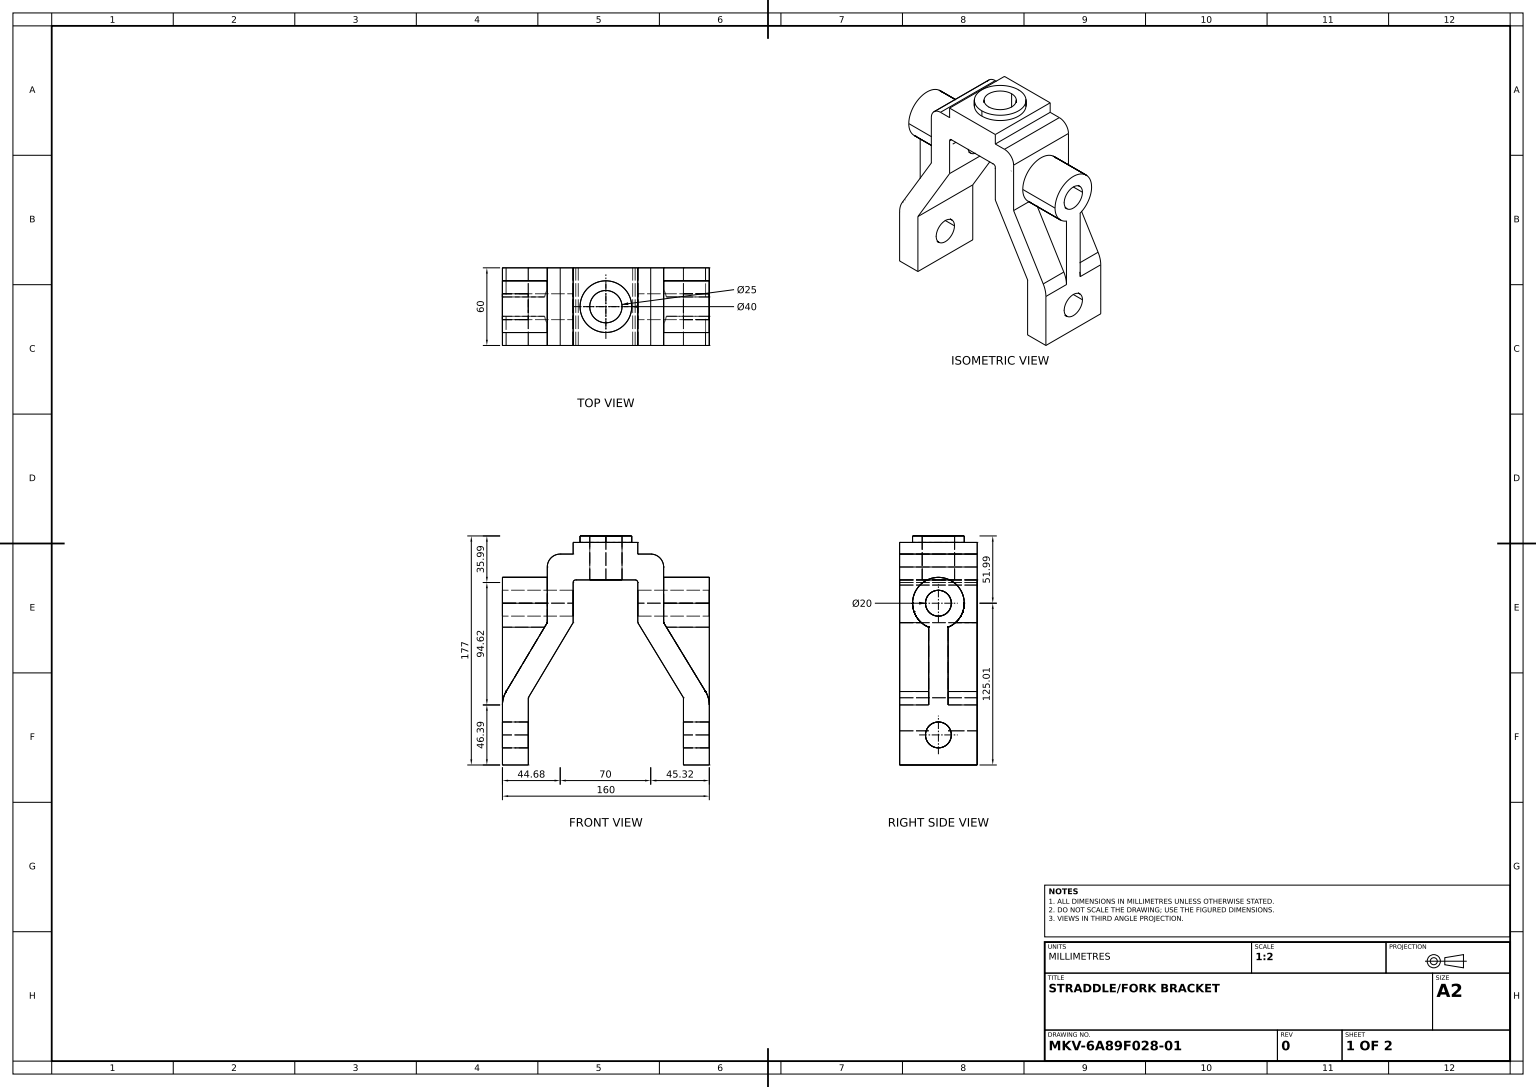
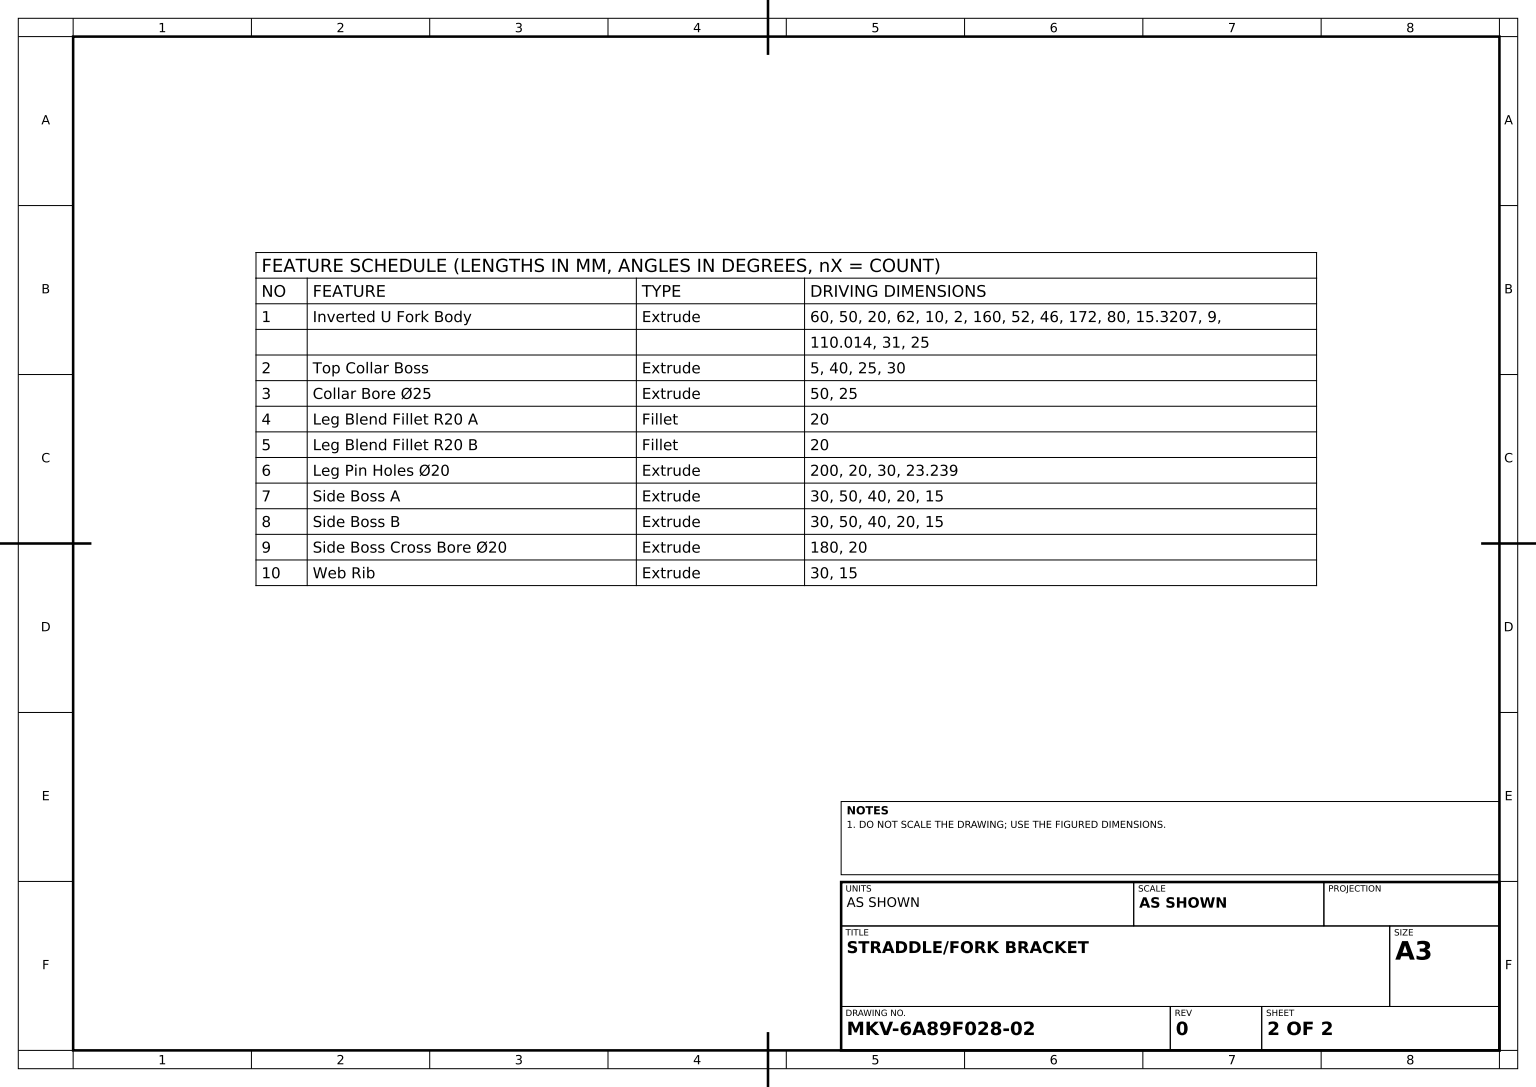
from build123d import *

# Parameters (mm, degrees)
INVERTED_U_FORK_BODY_DEPTH    = 60
TOP_COLLAR_BOSS_SKETCH_R      = 20
TOP_COLLAR_BOSS_SKETCH_R_2    = 12.5
TOP_COLLAR_BOSS_DEPTH         = 5
COLLAR_START                  = -50
COLLAR_BORE_SKETCH_R          = 12.5
COLLAR_BORE_25_DEPTH          = 50
LEG_BLEND_FILLET_R20_A_R      = 20
LEG_BLEND_FILLET_R20_B_R      = 20
LEG_PIN_HOLE_SKETCH_R         = 10
LEG_PIN_HOLES_20_DEPTH        = 200
SIDE_BOSS_A_SKETCH_R          = 20
SIDE_BOSS_A_SKETCH_R_2        = 10
SIDE_BOSS_A_DEPTH             = 50
SIDE_START                    = -50
SIDE_BOSS_B_SKETCH_R          = 20
SIDE_BOSS_B_SKETCH_R_2        = 10
SIDE_BOSS_B_DEPTH             = 50
SIDE_START_2                  = -180
SIDE_BOSS_CROSS_BORE_SKETCH_R = 10
SIDE_BOSS_CROSS_BORE_20_DEPTH = 180
WEB_RIB_DEPTH                 = 7.5


with BuildPart() as part:
    # Fork Profile Sketch → Inverted U Fork Body (new body)
    with BuildSketch(Plane.XY):
        with BuildLine():
            Line((-25.320668346, 110.01352712), (-25.320668346, 141.01352712))
            ThreePointArc((-25.320668346, 141.01352712), (-24.734881908, 142.427740683), (-23.320668346, 143.01352712))
            Line((-23.320668346, 143.01352712), (22.679331654, 143.01352712))
            ThreePointArc((22.679331654, 143.01352712), (24.093545217, 142.427740683), (24.679331654, 141.01352712))
            Line((24.679331654, 141.01352712), (24.679331654, 110.01352712))
            Line((24.679331654, 110.01352712), (60, 52))
            Line((60, 52), (60, 0))
            Line((60, 0), (80, 0))
            Line((80, 0), (80, 52))
            Line((80, 52), (44.679331654, 110.01352712))
            Line((44.679331654, 110.01352712), (44.679331654, 153))
            ThreePointArc((44.679331654, 153), (41.750399466, 160.071067812), (34.679331654, 163))
            Line((34.679331654, 163), (24.679331654, 163))
            Line((24.679331654, 163), (24.679331654, 172))
            Line((24.679331654, 172), (10, 172))
            Line((10, 172), (-10, 172))
            Line((-10, 172), (-25.320668346, 172))
            Line((-25.320668346, 172), (-25.320668346, 163))
            Line((-25.320668346, 163), (-35.320668346, 163))
            ThreePointArc((-35.320668346, 163), (-42.391736158, 160.071067812), (-45.320668346, 153))
            Line((-45.320668346, 153), (-45.320668346, 110.01352712))
            Line((-45.320668346, 110.01352712), (-80, 52))
            Line((-80, 52), (-80, 0))
            Line((-80, 0), (-60, 0))
            Line((-60, 0), (-60, 52))
            Line((-60, 52), (-25.320668346, 110.01352712))
        make_face()
    extrude(amount=INVERTED_U_FORK_BODY_DEPTH)

    # Top Collar Boss Sketch → Top Collar Boss (add)
    with BuildSketch(Plane(origin=(0, 172, 0), x_dir=(1, 0, 0), z_dir=(0, 1, 0))):
        with Locations(Location((0, -30, 0), (0, 0, 270))):
            Circle(TOP_COLLAR_BOSS_SKETCH_R)
        with Locations(Location((0, -30, 0), (0, 0, 270))):
            Circle(TOP_COLLAR_BOSS_SKETCH_R_2, mode=Mode.SUBTRACT)
    extrude(amount=TOP_COLLAR_BOSS_DEPTH)

    # Collar Bore Sketch → Collar Bore Ø25 (cut)
    with BuildSketch(Plane(origin=(0, 172, 0), x_dir=(1, 0, 0), z_dir=(0, 1, 0)).offset(COLLAR_START)):
        with Locations(Location((0, -30, 0), (0, 0, 270))):
            Circle(COLLAR_BORE_SKETCH_R)
    extrude(amount=COLLAR_BORE_25_DEPTH, mode=Mode.SUBTRACT)

    # Leg Blend Fillet R20 A
    leg_blend_fillet_r20_a_edges = [part.edges().sort_by_distance(p)[0] for p in [
        (-80, 52, 30),
    ]]
    fillet(leg_blend_fillet_r20_a_edges, radius=LEG_BLEND_FILLET_R20_A_R)

    # Leg Blend Fillet R20 B
    leg_blend_fillet_r20_b_edges = [part.edges().sort_by_distance(p)[0] for p in [
        (80, 52, 30),
    ]]
    fillet(leg_blend_fillet_r20_b_edges, radius=LEG_BLEND_FILLET_R20_B_R)

    # Leg Pin Hole Sketch → Leg Pin Holes Ø20 (cut)
    with BuildSketch(Plane.ZY.offset(80)):
        with Locations((30, 23.238954536)):
            Circle(LEG_PIN_HOLE_SKETCH_R)
    extrude(amount=-LEG_PIN_HOLES_20_DEPTH, mode=Mode.SUBTRACT)

    # Side Boss A Sketch → Side Boss A (add)
    with BuildSketch(Plane(origin=(30, 0, 0), x_dir=(0, 0, -1), z_dir=(1, 0, 0))):
        with Locations(Location((-30, 125.01352712, 0), (0, 0, 228.590377891))):
            Circle(SIDE_BOSS_A_SKETCH_R)
        with Locations((-30, 125.01352712)):
            Circle(SIDE_BOSS_A_SKETCH_R_2, mode=Mode.SUBTRACT)
    extrude(amount=SIDE_BOSS_A_DEPTH)

    # Side Boss B Sketch → Side Boss B (add)
    with BuildSketch(Plane(origin=(-30, 0, 0), x_dir=(0, 0, -1), z_dir=(1, 0, 0)).offset(SIDE_START)):
        with Locations(Location((-30, 125.01352712, 0), (0, 0, 228.590377891))):
            Circle(SIDE_BOSS_B_SKETCH_R)
        with Locations((-30, 125.01352712)):
            Circle(SIDE_BOSS_B_SKETCH_R_2, mode=Mode.SUBTRACT)
    extrude(amount=SIDE_BOSS_B_DEPTH)

    # Side Boss Cross Bore Sketch → Side Boss Cross Bore Ø20 (cut)
    with BuildSketch(Plane(origin=(44.679331654, 0, 0), x_dir=(0, 0, -1), z_dir=(1, 0, 0)).offset(SIDE_START_2)):
        with Locations(Location((-30, 125.01352712, 0), (0, 0, 90))):
            Circle(SIDE_BOSS_CROSS_BORE_SKETCH_R)
    extrude(amount=SIDE_BOSS_CROSS_BORE_20_DEPTH, mode=Mode.SUBTRACT)

    # Web Rib Sketch → Web Rib (add, symmetric)
    with BuildSketch(Plane.XY.offset(30)):
        Polygon((-45.320668346, 110.01352712), (-80, 110.01352712), (-80, 46.477909073), align=None)
        Polygon((44.679331654, 110.01352712), (80, 110.01352712), (80, 46.390582944), align=None)
    extrude(amount=WEB_RIB_DEPTH, both=True)


solid = part.part
